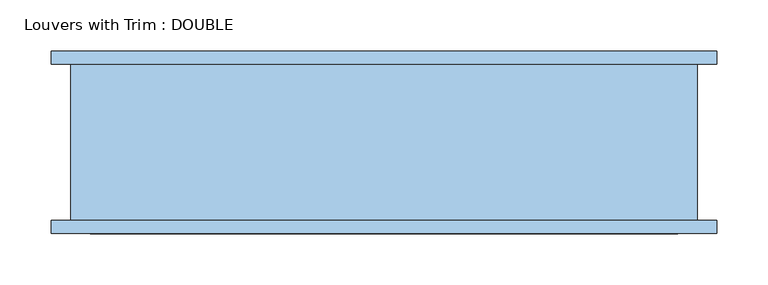
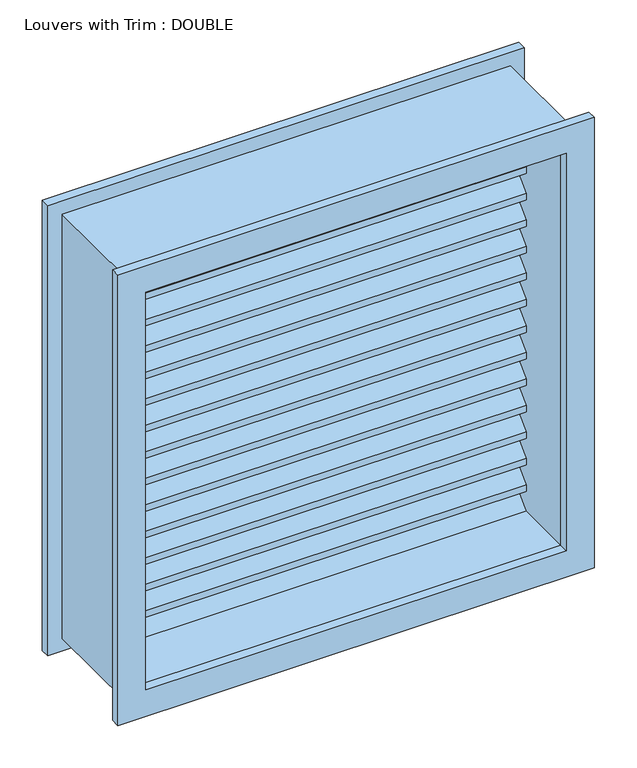
"""IFC4 building model written with IfcOpenShell, lengths in millimetres: window geometry, Louvers with Trim : DOUBLE."""

from ifc_helpers import new_model, si_unit, frame, origin, place, context, project, spatial, polyline, outline, extrude, source, transform, mapped, element, save


def louvers_with_trim_double_60c1390f(model_context):
    return source(origin(), model_context, "Body", "SweptSolid", [
        extrude(outline(polyline([(1543.05, -323.85), (895.35, -323.85), (895.35, 323.85), (1543.05, 323.85), (1543.05, -323.85)]), holes=[polyline([(1504.95, -285.75), (1504.95, 285.75), (933.45, 285.75), (933.45, -285.75), (1504.95, -285.75)])]), frame((0.0, 69.85, 0.0), z_axis=(0.0, 1.0, 0.0), x_axis=(0.0, 0.0, 1.0)), (0.0, 0.0, 1.0), 12.7),
        extrude(outline(polyline([(1543.05, 323.85), (1543.05, -323.85), (895.35, -323.85), (895.35, 323.85), (1543.05, 323.85)]), holes=[polyline([(1504.95, 285.75), (933.45, 285.75), (933.45, -285.75), (1504.95, -285.75), (1504.95, 285.75)])]), frame((0.0, -95.25, 0.0), z_axis=(0.0, 1.0, 0.0), x_axis=(0.0, 0.0, 1.0)), (0.0, 0.0, 1.0), 12.7),
        extrude(outline(polyline([(1524.0, 304.8), (1524.0, -304.8), (914.4, -304.8), (914.4, 304.8), (1524.0, 304.8)]), holes=[polyline([(1504.95, 285.75), (933.45, 285.75), (933.45, -285.75), (1504.95, -285.75), (1504.95, 285.75)])]), frame((0.0, -82.55, 0.0), z_axis=(0.0, 1.0, 0.0), x_axis=(0.0, 0.0, 1.0)), (0.0, 0.0, 1.0), 152.4),
        extrude(outline(polyline([(33.9289755, 969.3710245), (69.85, 933.45), (60.8697439, 933.45), (33.9289755, 960.3907684), (6.9882072, 933.45), (-1.992049, 933.45), (33.9289755, 969.3710245)])), frame((-285.75, 0.0, 0.0), z_axis=(1.0, 0.0, 0.0), x_axis=(0.0, 1.0, 0.0)), (0.0, 0.0, 1.0), 571.5),
        extrude(outline(polyline([(33.9289755, 1007.4710245), (69.85, 971.55), (69.85, 962.5697439), (33.9289755, 998.4907684), (-1.992049, 962.5697439), (-1.992049, 971.55), (33.9289755, 1007.4710245)])), frame((-285.75, 0.0, 0.0), z_axis=(1.0, 0.0, 0.0), x_axis=(0.0, 1.0, 0.0)), (0.0, 0.0, 1.0), 571.5),
        extrude(outline(polyline([(33.9289755, 1045.5710245), (69.85, 1009.65), (69.85, 1000.6697439), (33.9289755, 1036.5907684), (-1.992049, 1000.6697439), (-1.992049, 1009.65), (33.9289755, 1045.5710245)])), frame((-285.75, 0.0, 0.0), z_axis=(1.0, 0.0, 0.0), x_axis=(0.0, 1.0, 0.0)), (0.0, 0.0, 1.0), 571.5),
        extrude(outline(polyline([(33.9289755, 1083.6710245), (69.85, 1047.75), (69.85, 1038.7697439), (33.9289755, 1074.6907684), (-1.992049, 1038.7697439), (-1.992049, 1047.75), (33.9289755, 1083.6710245)])), frame((-285.75, 0.0, 0.0), z_axis=(1.0, 0.0, 0.0), x_axis=(0.0, 1.0, 0.0)), (0.0, 0.0, 1.0), 571.5),
        extrude(outline(polyline([(33.9289755, 1121.7710245), (69.85, 1085.85), (69.85, 1076.8697439), (33.9289755, 1112.7907684), (-1.992049, 1076.8697439), (-1.992049, 1085.85), (33.9289755, 1121.7710245)])), frame((-285.75, 0.0, 0.0), z_axis=(1.0, 0.0, 0.0), x_axis=(0.0, 1.0, 0.0)), (0.0, 0.0, 1.0), 571.5),
        extrude(outline(polyline([(33.9289755, 1159.8710245), (69.85, 1123.95), (69.85, 1114.9697439), (33.9289755, 1150.8907684), (-1.992049, 1114.9697439), (-1.992049, 1123.95), (33.9289755, 1159.8710245)])), frame((-285.75, 0.0, 0.0), z_axis=(1.0, 0.0, 0.0), x_axis=(0.0, 1.0, 0.0)), (0.0, 0.0, 1.0), 571.5),
        extrude(outline(polyline([(33.9289755, 1197.9710245), (69.85, 1162.05), (69.85, 1153.0697439), (33.9289755, 1188.9907684), (-1.992049, 1153.0697439), (-1.992049, 1162.05), (33.9289755, 1197.9710245)])), frame((-285.75, 0.0, 0.0), z_axis=(1.0, 0.0, 0.0), x_axis=(0.0, 1.0, 0.0)), (0.0, 0.0, 1.0), 571.5),
        extrude(outline(polyline([(33.9289755, 1236.0710245), (69.85, 1200.15), (69.85, 1191.1697439), (33.9289755, 1227.0907684), (-1.992049, 1191.1697439), (-1.992049, 1200.15), (33.9289755, 1236.0710245)])), frame((-285.75, 0.0, 0.0), z_axis=(1.0, 0.0, 0.0), x_axis=(0.0, 1.0, 0.0)), (0.0, 0.0, 1.0), 571.5),
        extrude(outline(polyline([(33.9289755, 1274.1710245), (69.85, 1238.25), (69.85, 1229.2697439), (33.9289755, 1265.1907684), (-1.992049, 1229.2697439), (-1.992049, 1238.25), (33.9289755, 1274.1710245)])), frame((-285.75, 0.0, 0.0), z_axis=(1.0, 0.0, 0.0), x_axis=(0.0, 1.0, 0.0)), (0.0, 0.0, 1.0), 571.5),
        extrude(outline(polyline([(33.9289755, 1312.2710245), (69.85, 1276.35), (69.85, 1267.3697439), (33.9289755, 1303.2907684), (-1.992049, 1267.3697439), (-1.992049, 1276.35), (33.9289755, 1312.2710245)])), frame((-285.75, 0.0, 0.0), z_axis=(1.0, 0.0, 0.0), x_axis=(0.0, 1.0, 0.0)), (0.0, 0.0, 1.0), 571.5),
        extrude(outline(polyline([(33.9289755, 1350.3710245), (69.85, 1314.45), (69.85, 1305.4697439), (33.9289755, 1341.3907684), (-1.992049, 1305.4697439), (-1.992049, 1314.45), (33.9289755, 1350.3710245)])), frame((-285.75, 0.0, 0.0), z_axis=(1.0, 0.0, 0.0), x_axis=(0.0, 1.0, 0.0)), (0.0, 0.0, 1.0), 571.5),
        extrude(outline(polyline([(33.9289755, 1388.4710245), (69.85, 1352.55), (69.85, 1343.5697439), (33.9289755, 1379.4907684), (-1.992049, 1343.5697439), (-1.992049, 1352.55), (33.9289755, 1388.4710245)])), frame((-285.75, 0.0, 0.0), z_axis=(1.0, 0.0, 0.0), x_axis=(0.0, 1.0, 0.0)), (0.0, 0.0, 1.0), 571.5),
        extrude(outline(polyline([(33.9289755, 1426.5710245), (69.85, 1390.65), (69.85, 1381.6697439), (33.9289755, 1417.5907684), (-1.992049, 1381.6697439), (-1.992049, 1390.65), (33.9289755, 1426.5710245)])), frame((-285.75, 0.0, 0.0), z_axis=(1.0, 0.0, 0.0), x_axis=(0.0, 1.0, 0.0)), (0.0, 0.0, 1.0), 571.5),
        extrude(outline(polyline([(33.9289755, 1464.6710245), (69.85, 1428.75), (69.85, 1419.7697439), (33.9289755, 1455.6907684), (-1.992049, 1419.7697439), (-1.992049, 1428.75), (33.9289755, 1464.6710245)])), frame((-285.75, 0.0, 0.0), z_axis=(1.0, 0.0, 0.0), x_axis=(0.0, 1.0, 0.0)), (0.0, 0.0, 1.0), 571.5),
        extrude(outline(polyline([(33.9289755, 1502.7710245), (69.85, 1466.85), (69.85, 1457.8697439), (33.9289755, 1493.7907684), (-1.992049, 1457.8697439), (-1.992049, 1466.85), (33.9289755, 1502.7710245)])), frame((-285.75, 0.0, 0.0), z_axis=(1.0, 0.0, 0.0), x_axis=(0.0, 1.0, 0.0)), (0.0, 0.0, 1.0), 571.5),
    ])


if __name__ == "__main__":
    model = new_model("IFC4")
    model_context = context("Model", 3, world=origin())
    ifc_project = project(units=[si_unit("LENGTHUNIT", "METRE", prefix="MILLI")], contexts=[model_context])
    site = spatial("IfcSite", under=ifc_project)
    building = spatial("IfcBuilding", under=site)
    placement = place(None, origin())
    louvers_with_trim_double_shape = louvers_with_trim_double_60c1390f(model_context)
    element("IfcWindow", 1, ObjectType="Louvers with Trim : DOUBLE", at=placement, inside=building, context=model_context, shape_type="MappedRepresentation", body=[
        mapped(louvers_with_trim_double_shape, transform((0.0, 0.0, 0.0), x_axis=(1.0, 0.0, 0.0), y_axis=(0.0, 1.0, 0.0), z_axis=(0.0, 0.0, 1.0))),
    ])
    save(model, "model.ifc")

# Revit data of these elements
# Type "Louvers with Trim : DOUBLE"
#   Type Mark = "28"
#   Construction Type Id = "GSP4R"
#   Assembly Code = "B20"
#   Analytic Construction = "1/8 in Pilkington single glazing"
#   Visual Light Transmittance = 0.9
#   Solar Heat Gain Coefficient = 0.78
#   Heat Transfer Coefficient (U) = 0.6496 BTU/(h·ft²·°F)
#   Default Sill Height = 3' - 0"
#   Trim Projection - Ext. = 0' - 0 1/2"
#   Trim Projection - Int. = 0' - 0 1/2"
#   Trim Width - Exterior = 0' - 1 1/2"
#   Trim Width - Interior = 0' - 1 1/2"
#   Width = 2' - 0"
#   Define Thermal Properties by = 1
#   Frame Material = Birch
#   Louver Material = Birch
#   Trim Exterior Material = Birch
#   Trim Interior Material = Birch
#   Wall Closure = (empty or 0)
# Element 1 (IfcWindow, "Louvers with Trim : DOUBLE")
#   Materials on its faces: "Birch"
# Materials
#   "Birch": class "Wood", colour RGB 224 178 126, transparency 0, Description = "Betula Alleghaniensis", Cost = 0
